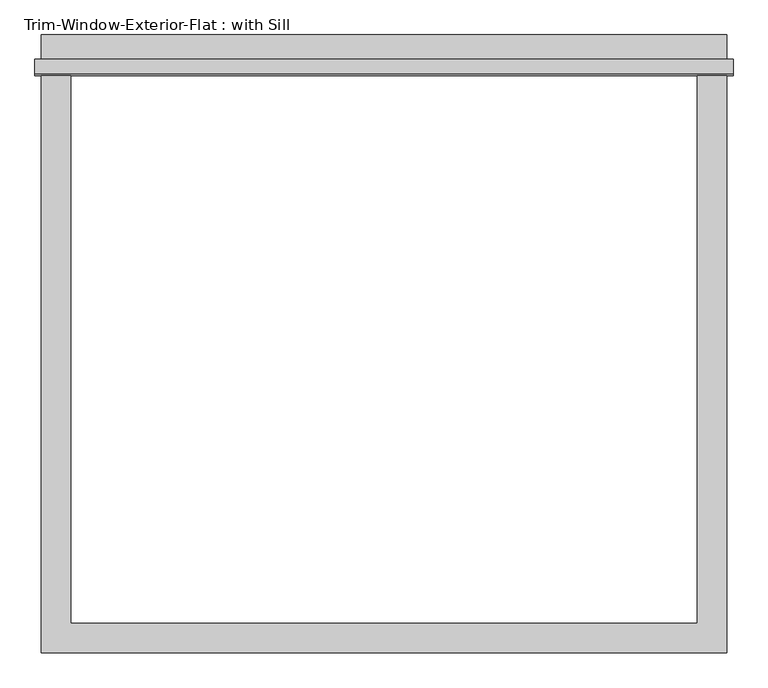
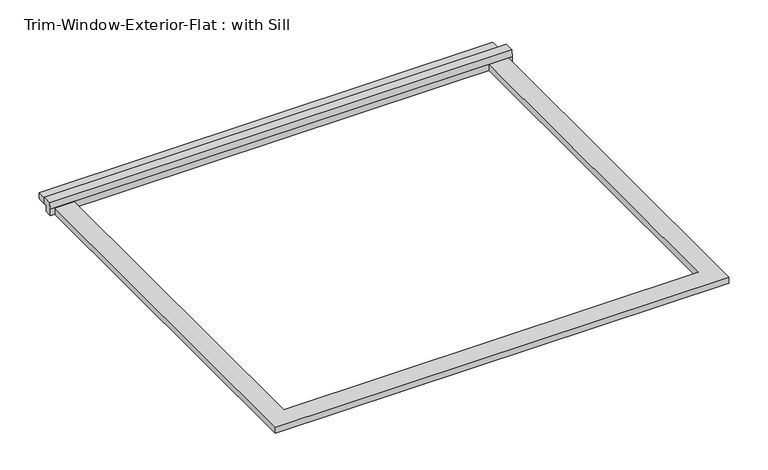
"""IFC4 building model written with IfcOpenShell, lengths in millimetres: proxy geometry, Trim-Window-Exterior-Flat : with Sill."""

from ifc_helpers import new_model, si_unit, frame, origin, origin_with_axes, place, context, project, spatial, polyline, outline, extrude, source, transform, mapped, element, save


def trim_window_exterior_flat_with_sill_e2e7eb1d(model_context):
    return source(origin(), model_context, "Body", "SweptSolid", [
        extrude(outline(polyline([(666.75, 1088.9823709), (-666.75, 1088.9823709), (-666.75, 1146.1323709), (666.75, 1146.1323709), (666.75, 1088.9823709)])), origin_with_axes(), (0.0, 0.0, 1.0), 19.05),
        extrude(outline(polyline([(1098.55, 38.1), (1098.55, 19.05), (1088.9823709, 19.05), (1088.9823709, 0.0), (1066.8, 0.0), (1066.8, 19.05), (1069.2580645, 38.1), (1098.55, 38.1)])), frame((-679.45, 0.0, 0.0), z_axis=(1.0, 0.0, 0.0), x_axis=(0.0, 1.0, 0.0)), (0.0, 0.0, 1.0), 1358.9),
        extrude(outline(polyline([(-666.75, -57.15), (-666.75, 1066.8), (-609.6, 1066.8), (-609.6, 0.0), (609.6, 0.0), (609.6, 1066.8), (666.75, 1066.8), (666.75, -57.15), (-666.75, -57.15)])), origin_with_axes(), (0.0, 0.0, 1.0), 19.05),
    ])


if __name__ == "__main__":
    model = new_model("IFC4")
    model_context = context("Model", 3, world=origin())
    ifc_project = project(units=[si_unit("LENGTHUNIT", "METRE", prefix="MILLI")], contexts=[model_context])
    site = spatial("IfcSite", under=ifc_project)
    building = spatial("IfcBuilding", under=site)
    placement = place(None, origin())
    trim_window_exterior_flat_with_sill_shape = trim_window_exterior_flat_with_sill_e2e7eb1d(model_context)
    element("IfcBuildingElementProxy", 1, Name="Trim-Window-Exterior-Flat : with Sill", ObjectType="Trim-Window-Exterior-Flat : with Sill", at=placement, inside=building, context=model_context, shape_type="MappedRepresentation", body=[
        mapped(trim_window_exterior_flat_with_sill_shape, transform((0.0, 0.0, 0.0), x_axis=(1.0, 0.0, 0.0), y_axis=(0.0, 1.0, 0.0), z_axis=(0.0, 0.0, 1.0))),
    ])
    save(model, "model.ifc")

# Revit data of these elements
# Type "Trim-Window-Exterior-Flat : with Sill"
#   Trim Width = 0' - 2 1/4"
#   Trim Thickness_Picture Frame = 0' - 1 1/4"
#   Trim Thickness_with Sill = 0' - 0 3/4"
#   Sill Thickness = 0' - 1 1/4"
#   Opening Width [instance default] = 2' - 0"
#   Opening Height [instance default] = 3' - 0"
#   Default Elevation = 4' - 0"
#   Sill = yes
#   Picture Frame = no
#   Trim Material [instance default] = none
# Element 1 (IfcBuildingElementProxy, "Trim-Window-Exterior-Flat : with Sill")
#   Opening Width = 4' - 0"
#   Opening Height = 3' - 6"
#   Trim Material = Clad - White
#   Materials on its faces: "Clad - White"
# Materials
#   "Clad - White": class "Wood", colour RGB 242 242 238, transparency 0, Cost = 0
